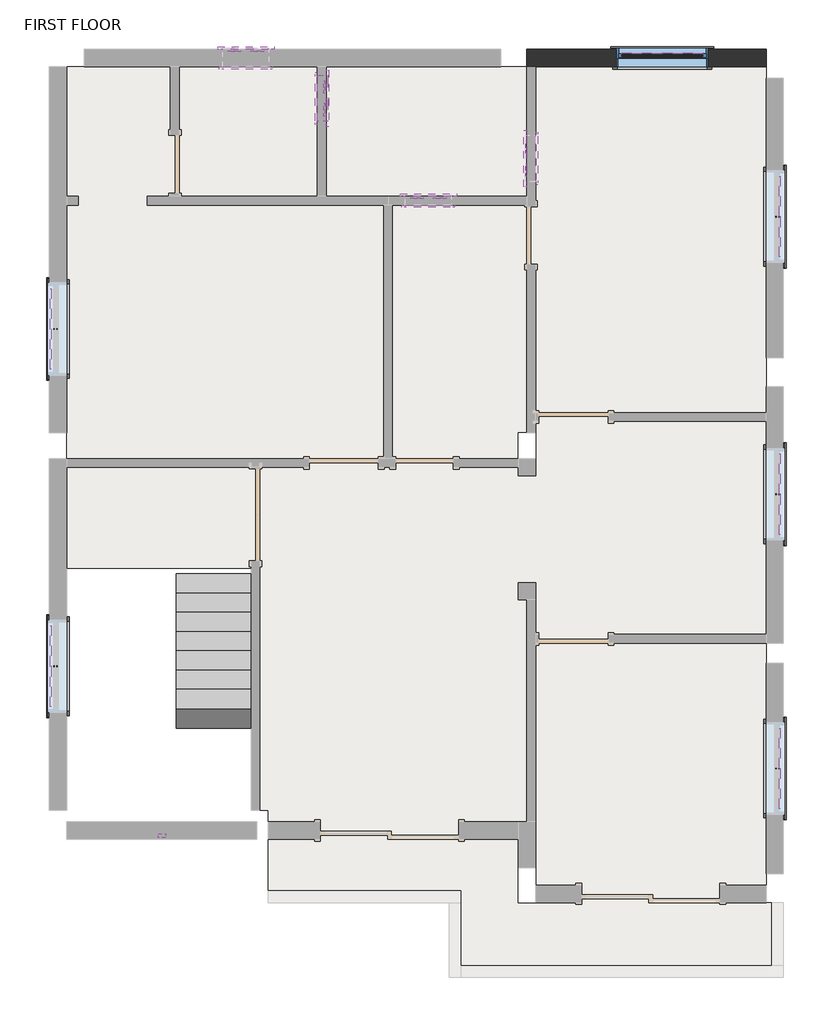
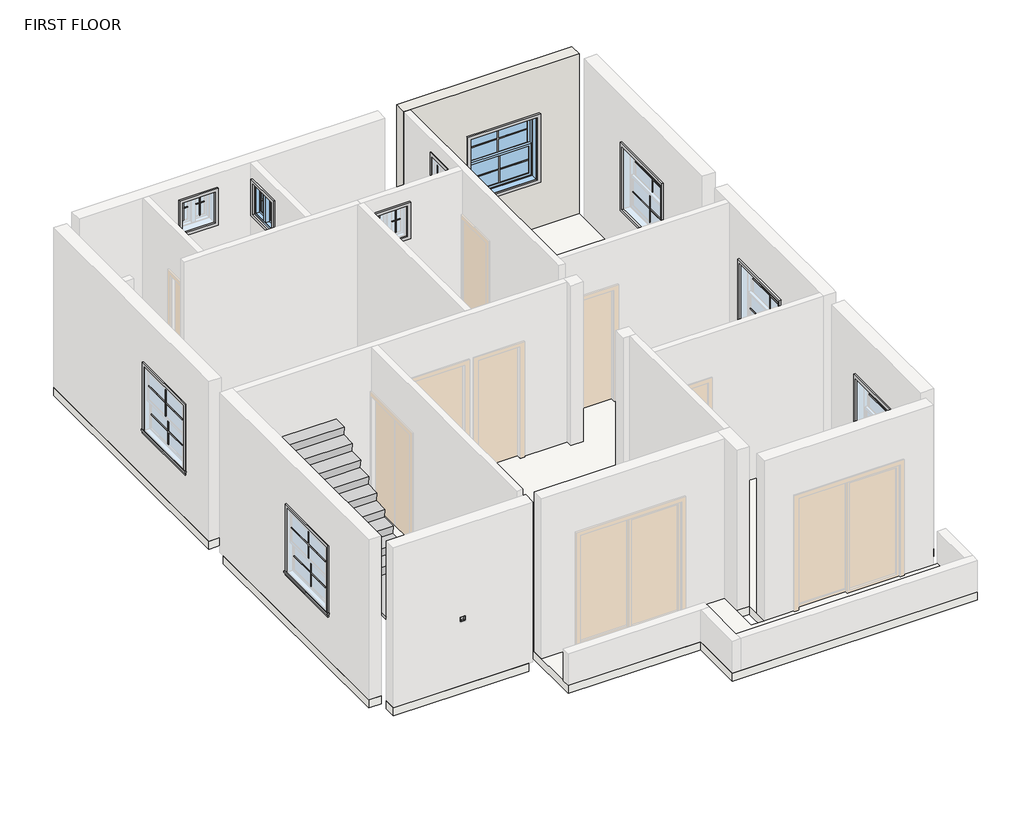
# One storey, part 2 of 2: 40 proxies, 2 windows, 1 light fixture, 1 slab, 1 stair flight, 1 wall.
"""IFC4 building model written with IfcOpenShell, lengths in millimetres."""

from ifc_helpers import new_model, si_unit, frame, origin, place, context, project, spatial, polyline, outline, extrude, faceted_brep, transform, mapped, element, save
from components import muntin_pattern_2x2_muntin_pattern_2x2_1e1a1b39, muntin_pattern_2x2_muntin_pattern_2x2_0961b91c, muntin_pattern_2x2_muntin_pattern_2x2_cae9449b, trim_window_exterior_flat_with_sill_7cfdd449, trim_window_exterior_flat_with_sill_858dc10d, trim_window_interior_flat_picture_frame_f1e0b15b, trim_window_interior_flat_picture_frame_3927330c, light_fixture_da35b629, window_casement_double_2_x2_e4709907, window_double_hung_4_x4_ec8efb0e

model = new_model("IFC4")

# Units and contexts
model_context = context("Model", 3, world=origin())
ifc_project = project(units=[si_unit("LENGTHUNIT", "METRE", prefix="MILLI")], contexts=[model_context])

# Site, building, storey
site = spatial("IfcSite", under=ifc_project)
building = spatial("IfcBuilding", under=site)
storey = spatial("IfcBuildingStorey", under=building, Name="FIRST FLOOR", Elevation=3200.4)

# Proxies
placement = place(None, origin())
muntin_pattern_2x2_muntin_pattern_2x2_shape = muntin_pattern_2x2_muntin_pattern_2x2_1e1a1b39(model_context)
element("IfcBuildingElementProxy", 1, Name="Muntin Pattern_2x2 : Muntin Pattern_2x2", ObjectType="Muntin Pattern_2x2 : Muntin Pattern_2x2", at=placement, inside=storey, context=model_context, shape_type="MappedRepresentation", body=[
    mapped(muntin_pattern_2x2_muntin_pattern_2x2_shape, transform((-12856.4959734, 734.3170657, 4746.625), x_axis=(0.0, 1.0, 0.0), y_axis=(-1.0, 0.0, 0.0), z_axis=(0.0, 0.0, 1.0))),
])
element("IfcBuildingElementProxy", 2, Name="Muntin Pattern_2x2 : Muntin Pattern_2x2", ObjectType="Muntin Pattern_2x2 : Muntin Pattern_2x2", at=placement, inside=storey, context=model_context, shape_type="MappedRepresentation", body=[
    mapped(muntin_pattern_2x2_muntin_pattern_2x2_shape, transform((-12812.0459734, 734.3170657, 4191.0), x_axis=(0.0, 1.0, 0.0), y_axis=(-1.0, 0.0, 0.0), z_axis=(0.0, 0.0, 1.0))),
])
element("IfcBuildingElementProxy", 3, Name="Muntin Pattern_2x2 : Muntin Pattern_2x2", ObjectType="Muntin Pattern_2x2 : Muntin Pattern_2x2", at=placement, inside=storey, context=model_context, shape_type="MappedRepresentation", body=[
    mapped(muntin_pattern_2x2_muntin_pattern_2x2_shape, transform((-12856.4959734, 5192.0170657, 4746.625), x_axis=(0.0, 1.0, 0.0), y_axis=(-1.0, 0.0, 0.0), z_axis=(0.0, 0.0, 1.0))),
])
element("IfcBuildingElementProxy", 4, Name="Muntin Pattern_2x2 : Muntin Pattern_2x2", ObjectType="Muntin Pattern_2x2 : Muntin Pattern_2x2", at=placement, inside=storey, context=model_context, shape_type="MappedRepresentation", body=[
    mapped(muntin_pattern_2x2_muntin_pattern_2x2_shape, transform((-12812.0459734, 5192.0170657, 4191.0), x_axis=(0.0, 1.0, 0.0), y_axis=(-1.0, 0.0, 0.0), z_axis=(0.0, 0.0, 1.0))),
])
element("IfcBuildingElementProxy", 5, Name="Muntin Pattern_2x2 : Muntin Pattern_2x2", ObjectType="Muntin Pattern_2x2 : Muntin Pattern_2x2", at=placement, inside=storey, context=model_context, shape_type="MappedRepresentation", body=[
    mapped(muntin_pattern_2x2_muntin_pattern_2x2_shape, transform((-4788.8209734, 8852.7920657, 4746.625), x_axis=(1.0, 0.0, 0.0), y_axis=(0.0, 1.0, 0.0), z_axis=(0.0, 0.0, 1.0))),
])
element("IfcBuildingElementProxy", 6, Name="Muntin Pattern_2x2 : Muntin Pattern_2x2", ObjectType="Muntin Pattern_2x2 : Muntin Pattern_2x2", at=placement, inside=storey, context=model_context, shape_type="MappedRepresentation", body=[
    mapped(muntin_pattern_2x2_muntin_pattern_2x2_shape, transform((-4788.8209734, 8808.3420657, 4191.0), x_axis=(1.0, 0.0, 0.0), y_axis=(0.0, 1.0, 0.0), z_axis=(0.0, 0.0, 1.0))),
])
element("IfcBuildingElementProxy", 7, Name="Muntin Pattern_2x2 : Muntin Pattern_2x2", ObjectType="Muntin Pattern_2x2 : Muntin Pattern_2x2", at=placement, inside=storey, context=model_context, shape_type="MappedRepresentation", body=[
    mapped(muntin_pattern_2x2_muntin_pattern_2x2_shape, transform((-3223.5459734, 6677.9170657, 4746.625), x_axis=(0.0, -1.0, 0.0), y_axis=(1.0, 0.0, 0.0), z_axis=(0.0, 0.0, 1.0))),
])
element("IfcBuildingElementProxy", 8, Name="Muntin Pattern_2x2 : Muntin Pattern_2x2", ObjectType="Muntin Pattern_2x2 : Muntin Pattern_2x2", at=placement, inside=storey, context=model_context, shape_type="MappedRepresentation", body=[
    mapped(muntin_pattern_2x2_muntin_pattern_2x2_shape, transform((-3267.9959734, 6677.9170657, 4191.0), x_axis=(0.0, -1.0, 0.0), y_axis=(1.0, 0.0, 0.0), z_axis=(0.0, 0.0, 1.0))),
])
element("IfcBuildingElementProxy", 9, Name="Muntin Pattern_2x2 : Muntin Pattern_2x2", ObjectType="Muntin Pattern_2x2 : Muntin Pattern_2x2", at=placement, inside=storey, context=model_context, shape_type="MappedRepresentation", body=[
    mapped(muntin_pattern_2x2_muntin_pattern_2x2_shape, transform((-3223.5459734, 3007.6170657, 4746.625), x_axis=(0.0, -1.0, 0.0), y_axis=(1.0, 0.0, 0.0), z_axis=(0.0, 0.0, 1.0))),
])
element("IfcBuildingElementProxy", 10, Name="Muntin Pattern_2x2 : Muntin Pattern_2x2", ObjectType="Muntin Pattern_2x2 : Muntin Pattern_2x2", at=placement, inside=storey, context=model_context, shape_type="MappedRepresentation", body=[
    mapped(muntin_pattern_2x2_muntin_pattern_2x2_shape, transform((-3267.9959734, 3007.6170657, 4191.0), x_axis=(0.0, -1.0, 0.0), y_axis=(1.0, 0.0, 0.0), z_axis=(0.0, 0.0, 1.0))),
])
element("IfcBuildingElementProxy", 11, Name="Muntin Pattern_2x2 : Muntin Pattern_2x2", ObjectType="Muntin Pattern_2x2 : Muntin Pattern_2x2", at=placement, inside=storey, context=model_context, shape_type="MappedRepresentation", body=[
    mapped(muntin_pattern_2x2_muntin_pattern_2x2_shape, transform((-3223.5459734, -618.2329343, 4746.625), x_axis=(0.0, -1.0, 0.0), y_axis=(1.0, 0.0, 0.0), z_axis=(0.0, 0.0, 1.0))),
])
element("IfcBuildingElementProxy", 12, Name="Muntin Pattern_2x2 : Muntin Pattern_2x2", ObjectType="Muntin Pattern_2x2 : Muntin Pattern_2x2", at=placement, inside=storey, context=model_context, shape_type="MappedRepresentation", body=[
    mapped(muntin_pattern_2x2_muntin_pattern_2x2_shape, transform((-3267.9959734, -618.2329343, 4191.0), x_axis=(0.0, -1.0, 0.0), y_axis=(1.0, 0.0, 0.0), z_axis=(0.0, 0.0, 1.0))),
])
muntin_pattern_2x2_muntin_pattern_2x2_2_shape = muntin_pattern_2x2_muntin_pattern_2x2_0961b91c(model_context)
element("IfcBuildingElementProxy", 13, Name="Muntin Pattern_2x2 : Muntin Pattern_2x2", ObjectType="Muntin Pattern_2x2 : Muntin Pattern_2x2", at=placement, inside=storey, context=model_context, shape_type="MappedRepresentation", body=[
    mapped(muntin_pattern_2x2_muntin_pattern_2x2_2_shape, transform((-8032.0834734, 6935.0920657, 5403.85), x_axis=(1.0, 0.0, 0.0), y_axis=(0.0, 1.0, 0.0), z_axis=(0.0, 0.0, 1.0))),
])
element("IfcBuildingElementProxy", 14, Name="Muntin Pattern_2x2 : Muntin Pattern_2x2", ObjectType="Muntin Pattern_2x2 : Muntin Pattern_2x2", at=placement, inside=storey, context=model_context, shape_type="MappedRepresentation", body=[
    mapped(muntin_pattern_2x2_muntin_pattern_2x2_2_shape, transform((-9243.3459734, 8390.8295657, 5403.85), x_axis=(0.0, -1.0, 0.0), y_axis=(1.0, 0.0, 0.0), z_axis=(0.0, 0.0, 1.0))),
])
element("IfcBuildingElementProxy", 15, Name="Muntin Pattern_2x2 : Muntin Pattern_2x2", ObjectType="Muntin Pattern_2x2 : Muntin Pattern_2x2", at=placement, inside=storey, context=model_context, shape_type="MappedRepresentation", body=[
    mapped(muntin_pattern_2x2_muntin_pattern_2x2_2_shape, transform((-10445.0834734, 8878.1920657, 5403.85), x_axis=(1.0, 0.0, 0.0), y_axis=(0.0, 1.0, 0.0), z_axis=(0.0, 0.0, 1.0))),
])
element("IfcBuildingElementProxy", 16, Name="Muntin Pattern_2x2 : Muntin Pattern_2x2", ObjectType="Muntin Pattern_2x2 : Muntin Pattern_2x2", at=placement, inside=storey, context=model_context, shape_type="MappedRepresentation", body=[
    mapped(muntin_pattern_2x2_muntin_pattern_2x2_2_shape, transform((-6569.9959734, 7295.4545657, 5403.85), x_axis=(0.0, 1.0, 0.0), y_axis=(-1.0, 0.0, 0.0), z_axis=(0.0, 0.0, 1.0))),
])
muntin_pattern_2x2_muntin_pattern_2x2_3_shape = muntin_pattern_2x2_muntin_pattern_2x2_cae9449b(model_context)
element("IfcBuildingElementProxy", 17, Name="Muntin Pattern_2x2 : Muntin Pattern_2x2", ObjectType="Muntin Pattern_2x2 : Muntin Pattern_2x2", at=placement, inside=storey, context=model_context, shape_type="MappedRepresentation", body=[
    mapped(muntin_pattern_2x2_muntin_pattern_2x2_3_shape, transform((-7730.4584734, 6935.0920657, 5403.85), x_axis=(-1.0, 0.0, 0.0), y_axis=(0.0, -1.0, 0.0), z_axis=(0.0, 0.0, 1.0))),
])
element("IfcBuildingElementProxy", 18, Name="Muntin Pattern_2x2 : Muntin Pattern_2x2", ObjectType="Muntin Pattern_2x2 : Muntin Pattern_2x2", at=placement, inside=storey, context=model_context, shape_type="MappedRepresentation", body=[
    mapped(muntin_pattern_2x2_muntin_pattern_2x2_3_shape, transform((-9243.3459734, 8089.2045657, 5403.85), x_axis=(0.0, 1.0, 0.0), y_axis=(-1.0, 0.0, 0.0), z_axis=(0.0, 0.0, 1.0))),
])
element("IfcBuildingElementProxy", 19, Name="Muntin Pattern_2x2 : Muntin Pattern_2x2", ObjectType="Muntin Pattern_2x2 : Muntin Pattern_2x2", at=placement, inside=storey, context=model_context, shape_type="MappedRepresentation", body=[
    mapped(muntin_pattern_2x2_muntin_pattern_2x2_3_shape, transform((-10143.4584734, 8878.1920657, 5403.85), x_axis=(-1.0, 0.0, 0.0), y_axis=(0.0, -1.0, 0.0), z_axis=(0.0, 0.0, 1.0))),
])
element("IfcBuildingElementProxy", 20, Name="Muntin Pattern_2x2 : Muntin Pattern_2x2", ObjectType="Muntin Pattern_2x2 : Muntin Pattern_2x2", at=placement, inside=storey, context=model_context, shape_type="MappedRepresentation", body=[
    mapped(muntin_pattern_2x2_muntin_pattern_2x2_3_shape, transform((-6569.9959734, 7597.0795657, 5403.85), x_axis=(0.0, -1.0, 0.0), y_axis=(1.0, 0.0, 0.0), z_axis=(0.0, 0.0, 1.0))),
])
trim_window_exterior_flat_with_sill_shape = trim_window_exterior_flat_with_sill_7cfdd449(model_context)
element("IfcBuildingElementProxy", 21, Name="Trim-Window-Exterior-Flat : with Sill", ObjectType="Trim-Window-Exterior-Flat : with Sill", at=placement, inside=storey, context=model_context, shape_type="MappedRepresentation", body=[
    mapped(trim_window_exterior_flat_with_sill_shape, transform((-12891.4209734, 734.3170657, 5334.0), x_axis=(0.0, -1.0, 0.0), y_axis=(0.0, 0.0, 1.0), z_axis=(-1.0, 0.0, 0.0))),
])
element("IfcBuildingElementProxy", 22, Name="Trim-Window-Exterior-Flat : with Sill", ObjectType="Trim-Window-Exterior-Flat : with Sill", at=placement, inside=storey, context=model_context, shape_type="MappedRepresentation", body=[
    mapped(trim_window_exterior_flat_with_sill_shape, transform((-12891.4209734, 5192.0170657, 5334.0), x_axis=(0.0, -1.0, 0.0), y_axis=(0.0, 0.0, 1.0), z_axis=(-1.0, 0.0, 0.0))),
])
element("IfcBuildingElementProxy", 23, Name="Trim-Window-Exterior-Flat : with Sill", ObjectType="Trim-Window-Exterior-Flat : with Sill", at=placement, inside=storey, context=model_context, shape_type="MappedRepresentation", body=[
    mapped(trim_window_exterior_flat_with_sill_shape, transform((-4788.8209734, 8887.7170657, 5334.0), x_axis=(-1.0, 0.0, 0.0), y_axis=(0.0, 0.0, 1.0), z_axis=(0.0, 1.0, 0.0))),
])
element("IfcBuildingElementProxy", 24, Name="Trim-Window-Exterior-Flat : with Sill", ObjectType="Trim-Window-Exterior-Flat : with Sill", at=placement, inside=storey, context=model_context, shape_type="MappedRepresentation", body=[
    mapped(trim_window_exterior_flat_with_sill_shape, transform((-3188.6209734, 6677.9170657, 5334.0), x_axis=(0.0, 1.0, 0.0), y_axis=(0.0, 0.0, 1.0), z_axis=(1.0, 0.0, 0.0))),
])
element("IfcBuildingElementProxy", 25, Name="Trim-Window-Exterior-Flat : with Sill", ObjectType="Trim-Window-Exterior-Flat : with Sill", at=placement, inside=storey, context=model_context, shape_type="MappedRepresentation", body=[
    mapped(trim_window_exterior_flat_with_sill_shape, transform((-3188.6209734, 3007.6170657, 5334.0), x_axis=(0.0, 1.0, 0.0), y_axis=(0.0, 0.0, 1.0), z_axis=(1.0, 0.0, 0.0))),
])
element("IfcBuildingElementProxy", 26, Name="Trim-Window-Exterior-Flat : with Sill", ObjectType="Trim-Window-Exterior-Flat : with Sill", at=placement, inside=storey, context=model_context, shape_type="MappedRepresentation", body=[
    mapped(trim_window_exterior_flat_with_sill_shape, transform((-3188.6209734, -618.2329343, 5334.0), x_axis=(0.0, 1.0, 0.0), y_axis=(0.0, 0.0, 1.0), z_axis=(1.0, 0.0, 0.0))),
])
trim_window_exterior_flat_with_sill_2_shape = trim_window_exterior_flat_with_sill_858dc10d(model_context)
element("IfcBuildingElementProxy", 27, Name="Trim-Window-Exterior-Flat : with Sill", ObjectType="Trim-Window-Exterior-Flat : with Sill", at=placement, inside=storey, context=model_context, shape_type="MappedRepresentation", body=[
    mapped(trim_window_exterior_flat_with_sill_2_shape, transform((-7881.2709734, 6944.6170657, 5943.6), x_axis=(-1.0, 0.0, 0.0), y_axis=(0.0, 0.0, 1.0), z_axis=(0.0, 1.0, 0.0))),
])
element("IfcBuildingElementProxy", 28, Name="Trim-Window-Exterior-Flat : with Sill", ObjectType="Trim-Window-Exterior-Flat : with Sill", at=placement, inside=storey, context=model_context, shape_type="MappedRepresentation", body=[
    mapped(trim_window_exterior_flat_with_sill_2_shape, transform((-9233.8209734, 8240.0170657, 5943.6), x_axis=(0.0, 1.0, 0.0), y_axis=(0.0, 0.0, 1.0), z_axis=(1.0, 0.0, 0.0))),
])
element("IfcBuildingElementProxy", 29, Name="Trim-Window-Exterior-Flat : with Sill", ObjectType="Trim-Window-Exterior-Flat : with Sill", at=placement, inside=storey, context=model_context, shape_type="MappedRepresentation", body=[
    mapped(trim_window_exterior_flat_with_sill_2_shape, transform((-10294.2709734, 8887.7170657, 5943.6), x_axis=(-1.0, 0.0, 0.0), y_axis=(0.0, 0.0, 1.0), z_axis=(0.0, 1.0, 0.0))),
])
element("IfcBuildingElementProxy", 30, Name="Trim-Window-Exterior-Flat : with Sill", ObjectType="Trim-Window-Exterior-Flat : with Sill", at=placement, inside=storey, context=model_context, shape_type="MappedRepresentation", body=[
    mapped(trim_window_exterior_flat_with_sill_2_shape, transform((-6579.5209734, 7446.2670657, 5943.6), x_axis=(0.0, -1.0, 0.0), y_axis=(0.0, 0.0, 1.0), z_axis=(-1.0, 0.0, 0.0))),
])
trim_window_interior_flat_picture_frame_shape = trim_window_interior_flat_picture_frame_f1e0b15b(model_context)
element("IfcBuildingElementProxy", 31, Name="Trim-Window-Interior-Flat : Picture Frame", ObjectType="Trim-Window-Interior-Flat : Picture Frame", at=placement, inside=storey, context=model_context, shape_type="MappedRepresentation", body=[
    mapped(trim_window_interior_flat_picture_frame_shape, transform((-12662.8209734, 734.3170657, 5334.0), x_axis=(0.0, 1.0, 0.0), y_axis=(0.0, 0.0, 1.0), z_axis=(1.0, 0.0, 0.0))),
])
element("IfcBuildingElementProxy", 32, Name="Trim-Window-Interior-Flat : Picture Frame", ObjectType="Trim-Window-Interior-Flat : Picture Frame", at=placement, inside=storey, context=model_context, shape_type="MappedRepresentation", body=[
    mapped(trim_window_interior_flat_picture_frame_shape, transform((-12662.8209734, 5192.0170657, 5334.0), x_axis=(0.0, 1.0, 0.0), y_axis=(0.0, 0.0, 1.0), z_axis=(1.0, 0.0, 0.0))),
])
element("IfcBuildingElementProxy", 33, Name="Trim-Window-Interior-Flat : Picture Frame", ObjectType="Trim-Window-Interior-Flat : Picture Frame", at=placement, inside=storey, context=model_context, shape_type="MappedRepresentation", body=[
    mapped(trim_window_interior_flat_picture_frame_shape, transform((-4788.8209734, 8659.1170657, 5334.0), x_axis=(1.0, 0.0, 0.0), y_axis=(0.0, 0.0, 1.0), z_axis=(0.0, -1.0, 0.0))),
])
element("IfcBuildingElementProxy", 34, Name="Trim-Window-Interior-Flat : Picture Frame", ObjectType="Trim-Window-Interior-Flat : Picture Frame", at=placement, inside=storey, context=model_context, shape_type="MappedRepresentation", body=[
    mapped(trim_window_interior_flat_picture_frame_shape, transform((-3417.2209734, 6677.9170657, 5334.0), x_axis=(0.0, -1.0, 0.0), y_axis=(0.0, 0.0, 1.0), z_axis=(-1.0, 0.0, 0.0))),
])
element("IfcBuildingElementProxy", 35, Name="Trim-Window-Interior-Flat : Picture Frame", ObjectType="Trim-Window-Interior-Flat : Picture Frame", at=placement, inside=storey, context=model_context, shape_type="MappedRepresentation", body=[
    mapped(trim_window_interior_flat_picture_frame_shape, transform((-3417.2209734, 3007.6170657, 5334.0), x_axis=(0.0, -1.0, 0.0), y_axis=(0.0, 0.0, 1.0), z_axis=(-1.0, 0.0, 0.0))),
])
element("IfcBuildingElementProxy", 36, Name="Trim-Window-Interior-Flat : Picture Frame", ObjectType="Trim-Window-Interior-Flat : Picture Frame", at=placement, inside=storey, context=model_context, shape_type="MappedRepresentation", body=[
    mapped(trim_window_interior_flat_picture_frame_shape, transform((-3417.2209734, -618.2329343, 5334.0), x_axis=(0.0, -1.0, 0.0), y_axis=(0.0, 0.0, 1.0), z_axis=(-1.0, 0.0, 0.0))),
])
trim_window_interior_flat_picture_frame_2_shape = trim_window_interior_flat_picture_frame_3927330c(model_context)
element("IfcBuildingElementProxy", 37, Name="Trim-Window-Interior-Flat : Picture Frame", ObjectType="Trim-Window-Interior-Flat : Picture Frame", at=placement, inside=storey, context=model_context, shape_type="MappedRepresentation", body=[
    mapped(trim_window_interior_flat_picture_frame_2_shape, transform((-7881.2709734, 6830.3170657, 5943.6), x_axis=(1.0, 0.0, 0.0), y_axis=(0.0, 0.0, 1.0), z_axis=(0.0, -1.0, 0.0))),
])
element("IfcBuildingElementProxy", 38, Name="Trim-Window-Interior-Flat : Picture Frame", ObjectType="Trim-Window-Interior-Flat : Picture Frame", at=placement, inside=storey, context=model_context, shape_type="MappedRepresentation", body=[
    mapped(trim_window_interior_flat_picture_frame_2_shape, transform((-9348.1209734, 8240.0170657, 5943.6), x_axis=(0.0, -1.0, 0.0), y_axis=(0.0, 0.0, 1.0), z_axis=(-1.0, 0.0, 0.0))),
])
element("IfcBuildingElementProxy", 39, Name="Trim-Window-Interior-Flat : Picture Frame", ObjectType="Trim-Window-Interior-Flat : Picture Frame", at=placement, inside=storey, context=model_context, shape_type="MappedRepresentation", body=[
    mapped(trim_window_interior_flat_picture_frame_2_shape, transform((-10294.2709734, 8659.1170657, 5943.6), x_axis=(1.0, 0.0, 0.0), y_axis=(0.0, 0.0, 1.0), z_axis=(0.0, -1.0, 0.0))),
])
element("IfcBuildingElementProxy", 40, Name="Trim-Window-Interior-Flat : Picture Frame", ObjectType="Trim-Window-Interior-Flat : Picture Frame", at=placement, inside=storey, context=model_context, shape_type="MappedRepresentation", body=[
    mapped(trim_window_interior_flat_picture_frame_2_shape, transform((-6465.2209734, 7446.2670657, 5943.6), x_axis=(0.0, 1.0, 0.0), y_axis=(0.0, 0.0, 1.0), z_axis=(1.0, 0.0, 0.0))),
])

# Light fixture
light_fixture_shape = light_fixture_da35b629(model_context)
element("IfcLightFixture", 41, at=placement, inside=storey, context=model_context, shape_type="MappedRepresentation", body=[
    mapped(light_fixture_shape, transform((-11441.8766361, -1437.3829343, 2452.7878889), x_axis=(-1.0, 0.0, 0.0), y_axis=(0.0, -1.0, 0.0), z_axis=(0.0, 0.0, 1.0))),
])

# Slab
element("IfcSlab", 42, ObjectType="6\"", at=placement, inside=storey, context=model_context, shape_type="SweptSolid", body=[
    extrude(outline(polyline([(-3188.6209734, -3380.4829343), (-7608.2209734, -3380.4829343), (-7608.2209734, -2389.8829343), (-9995.8209734, -2389.8829343), (-9995.8209734, -1170.6829343), (-10224.4209734, -1170.6829343), (-10224.4209734, 2029.7170657), (-12662.8209734, 2029.7170657), (-12662.8209734, -1170.6829343), (-12891.4209734, -1170.6829343), (-12891.4209734, 3363.2170657), (-12662.8209734, 3363.2170657), (-12662.8209734, 3820.4170657), (-12891.4209734, 3820.4170657), (-12891.4209734, 8659.1170657), (-12434.2209734, 8659.1170657), (-12434.2209734, 8887.7170657), (-6922.4209734, 8887.7170657), (-6922.4209734, 8659.1170657), (-6465.2209734, 8659.1170657), (-6465.2209734, 8887.7170657), (-3417.2209734, 8887.7170657), (-3417.2209734, 8506.7170657), (-3188.6209734, 8506.7170657), (-3188.6209734, 4811.0170657), (-3417.2209734, 4811.0170657), (-3417.2209734, 4430.0170657), (-3188.6209734, 4430.0170657), (-3188.6209734, 1153.4170657), (-3417.2209734, 1153.4170657), (-3417.2209734, 772.4170657), (-3188.6209734, 772.4170657), (-3188.6209734, -1746.9354412), (-3188.6209734, -2008.8829343), (-3417.2209734, -2008.8829343), (-3417.2209734, -2389.8829343), (-3188.6209734, -2389.8829343), (-3188.6209734, -3380.4829343)]), holes=[polyline([(-6693.8209734, -1932.6829343), (-6693.8209734, -2389.8829343), (-6465.2209734, -2389.8829343), (-6465.2209734, -1932.6829343), (-6693.8209734, -1932.6829343)]), polyline([(-6693.8209734, 3820.4170657), (-6693.8209734, 3363.2170657), (-6465.2209734, 3363.2170657), (-6465.2209734, 3820.4170657), (-6693.8209734, 3820.4170657)])]), frame((0.0, 0.0, 3048.0), z_axis=(0.0, 0.0, 1.0), x_axis=(1.0, 0.0, 0.0)), (0.0, 0.0, 1.0), 152.4),
    extrude(outline(polyline([(-12662.8209734, -1323.0829343), (-10224.4209734, -1323.0829343), (-10224.4209734, -1551.6829343), (-12662.8209734, -1551.6829343), (-12662.8209734, -1323.0829343)])), frame((0.0, 0.0, 3048.0), z_axis=(0.0, 0.0, 1.0), x_axis=(1.0, 0.0, 0.0)), (0.0, 0.0, 1.0), 152.4),
])

# Stair flight
element("IfcStairFlight", 43, ObjectType="3/4\" Nosing", at=placement, inside=storey, context=model_context, shape_type="Brep", body=[
    faceted_brep([(-10224.4209734, 1953.5170657, 3360.42), (-11215.0209734, 1953.5170657, 3360.42), (-11215.0209734, 1680.4670657, 3360.42), (-10224.4209734, 1680.4670657, 3360.42), (-10224.4209734, 1680.4670657, 3285.3690172), (-10224.4209734, 1815.3385215, 3200.4), (-10224.4209734, 1934.4670657, 3200.4), (-11215.0209734, 1934.4670657, 3200.4), (-11215.0209734, 1815.3385215, 3200.4), (-11215.0209734, 1680.4670657, 3285.3690172), (-10224.4209734, 1699.5170657, 3520.44), (-11215.0209734, 1699.5170657, 3520.44), (-11215.0209734, 1426.4670657, 3520.44), (-10224.4209734, 1426.4670657, 3520.44), (-10224.4209734, 1426.4670657, 3445.3890172), (-11215.0209734, 1426.4670657, 3445.3890172), (-10224.4209734, 1445.5170657, 3680.46), (-11215.0209734, 1445.5170657, 3680.46), (-11215.0209734, 1172.4670657, 3680.46), (-10224.4209734, 1172.4670657, 3680.46), (-10224.4209734, 1172.4670657, 3605.4090172), (-11215.0209734, 1172.4670657, 3605.4090172), (-10224.4209734, 1191.5170657, 3840.48), (-11215.0209734, 1191.5170657, 3840.48), (-11215.0209734, 918.4670657, 3840.48), (-10224.4209734, 918.4670657, 3840.48), (-10224.4209734, 918.4670657, 3765.4290172), (-11215.0209734, 918.4670657, 3765.4290172), (-10224.4209734, 937.5170657, 4000.5), (-11215.0209734, 937.5170657, 4000.5), (-11215.0209734, 664.4670657, 4000.5), (-10224.4209734, 664.4670657, 4000.5), (-10224.4209734, 664.4670657, 3925.4490172), (-11215.0209734, 664.4670657, 3925.4490172), (-10224.4209734, 683.5170657, 4160.52), (-11215.0209734, 683.5170657, 4160.52), (-11215.0209734, 410.4670657, 4160.52), (-10224.4209734, 410.4670657, 4160.52), (-10224.4209734, 410.4670657, 4085.4690172), (-11215.0209734, 410.4670657, 4085.4690172), (-10224.4209734, 429.5170657, 4320.54), (-11215.0209734, 429.5170657, 4320.54), (-11215.0209734, 156.4670657, 4320.54), (-10224.4209734, 156.4670657, 4320.54), (-10224.4209734, 156.4670657, 4245.4890172), (-11215.0209734, 156.4670657, 4245.4890172), (-10224.4209734, 175.5170657, 4480.56), (-11215.0209734, 175.5170657, 4480.56), (-11215.0209734, -97.5329343, 4480.56), (-10224.4209734, -97.5329343, 4480.56), (-10224.4209734, -97.5329343, 4405.5090172), (-11215.0209734, -97.5329343, 4405.5090172), (-10224.4209734, -78.4829343, 4640.58), (-11215.0209734, -78.4829343, 4640.58), (-11215.0209734, -351.5329343, 4640.58), (-10224.4209734, -351.5329343, 4640.58), (-10224.4209734, -351.5329343, 4565.5290172), (-11215.0209734, -623.8678277, 4737.1), (-11215.0209734, -340.0424581, 4737.1), (-12662.8209734, -313.4329343, 4800.6), (-12662.8209734, -1323.0829343, 4800.6), (-10224.4209734, -1323.0829343, 4800.6), (-10224.4209734, -623.8678277, 4800.6), (-10224.4209734, -332.4829343, 4800.6), (-11215.0209734, -332.4829343, 4800.6), (-11672.2209734, -332.4829343, 4800.6), (-11672.2209734, -313.4329343, 4800.6), (-12662.8209734, -313.4329343, 4737.1), (-12662.8209734, -1323.0829343, 4737.1), (-10224.4209734, -1323.0829343, 4737.1), (-10224.4209734, -623.8678277, 4737.1), (-11215.0209734, -332.4829343, 4737.1), (-11672.2209734, -332.4829343, 4737.1), (-11672.2209734, -313.4329343, 4737.1), (-12662.8209734, -332.4829343, 4960.62), (-11672.2209734, -332.4829343, 4960.62), (-11672.2209734, -295.0980409, 4960.62), (-11672.2209734, -59.4329343, 4960.62), (-12662.8209734, -59.4329343, 4960.62), (-12662.8209734, -295.0980409, 4960.62), (-12662.8209734, -59.4329343, 4885.5690172), (-12662.8209734, -295.0980409, 4737.1), (-11672.2209734, -295.0980409, 4737.1), (-11672.2209734, -59.4329343, 4885.5690172), (-12662.8209734, -78.4829343, 5120.64), (-11672.2209734, -78.4829343, 5120.64), (-11672.2209734, 194.5670657, 5120.64), (-12662.8209734, 194.5670657, 5120.64), (-12662.8209734, 194.5670657, 5045.5890172), (-11672.2209734, 194.5670657, 5045.5890172), (-12662.8209734, 175.5170657, 5280.66), (-11672.2209734, 175.5170657, 5280.66), (-11672.2209734, 448.5670657, 5280.66), (-12662.8209734, 448.5670657, 5280.66), (-12662.8209734, 448.5670657, 5205.6090172), (-11672.2209734, 448.5670657, 5205.6090172), (-12662.8209734, 429.5170657, 5440.68), (-11672.2209734, 429.5170657, 5440.68), (-11672.2209734, 702.5670657, 5440.68), (-12662.8209734, 702.5670657, 5440.68), (-12662.8209734, 702.5670657, 5365.6290172), (-11672.2209734, 702.5670657, 5365.6290172), (-12662.8209734, 683.5170657, 5600.7), (-11672.2209734, 683.5170657, 5600.7), (-11672.2209734, 956.5670657, 5600.7), (-12662.8209734, 956.5670657, 5600.7), (-12662.8209734, 956.5670657, 5525.6490172), (-11672.2209734, 956.5670657, 5525.6490172), (-12662.8209734, 937.5170657, 5760.72), (-11672.2209734, 937.5170657, 5760.72), (-11672.2209734, 1210.5670657, 5760.72), (-12662.8209734, 1210.5670657, 5760.72), (-12662.8209734, 1210.5670657, 5685.6690172), (-11672.2209734, 1210.5670657, 5685.6690172), (-12662.8209734, 1191.5170657, 5920.74), (-11672.2209734, 1191.5170657, 5920.74), (-11672.2209734, 1464.5670657, 5920.74), (-12662.8209734, 1464.5670657, 5920.74), (-12662.8209734, 1464.5670657, 5845.6890172), (-11672.2209734, 1464.5670657, 5845.6890172), (-12662.8209734, 1445.5170657, 6080.76), (-11672.2209734, 1445.5170657, 6080.76), (-11672.2209734, 1718.5670657, 6080.76), (-12662.8209734, 1718.5670657, 6080.76), (-12662.8209734, 1718.5670657, 6005.7090172), (-11672.2209734, 1718.5670657, 6005.7090172), (-12662.8209734, 1699.5170657, 6240.78), (-11672.2209734, 1699.5170657, 6240.78), (-11672.2209734, 1953.5170657, 6240.78), (-12662.8209734, 1953.5170657, 6240.78), (-12662.8209734, 1953.5170657, 6153.7275172), (-11672.2209734, 1953.5170657, 6153.7275172)], [[[0, 1, 2, 3]], [[0, 3, 4, 5, 6]], [[2, 1, 7, 8, 9]], [[10, 11, 12, 13]], [[10, 13, 14, 4, 3]], [[12, 11, 2, 9, 15]], [[16, 17, 18, 19]], [[16, 19, 20, 14, 13]], [[18, 17, 12, 15, 21]], [[22, 23, 24, 25]], [[22, 25, 26, 20, 19]], [[24, 23, 18, 21, 27]], [[28, 29, 30, 31]], [[28, 31, 32, 26, 25]], [[30, 29, 24, 27, 33]], [[34, 35, 36, 37]], [[34, 37, 38, 32, 31]], [[36, 35, 30, 33, 39]], [[40, 41, 42, 43]], [[40, 43, 44, 38, 37]], [[42, 41, 36, 39, 45]], [[46, 47, 48, 49]], [[46, 49, 50, 44, 43]], [[48, 47, 42, 45, 51]], [[52, 53, 54, 55]], [[52, 55, 56, 50, 49]], [[53, 48, 51, 57, 58, 54]], [[59, 60, 61, 62, 63, 64, 65, 66]], [[60, 59, 67, 68]], [[61, 60, 68, 69]], [[55, 63, 62, 61, 69, 70, 56]], [[64, 58, 71]], [[65, 64, 71, 72]], [[66, 65, 72, 73]], [[74, 75, 76, 77, 78, 79]], [[59, 74, 79, 78, 80, 81, 67]], [[75, 66, 73, 82, 83, 77, 76]], [[84, 85, 86, 87]], [[84, 87, 88, 80, 78]], [[86, 85, 77, 83, 89]], [[90, 91, 92, 93]], [[90, 93, 94, 88, 87]], [[92, 91, 86, 89, 95]], [[96, 97, 98, 99]], [[96, 99, 100, 94, 93]], [[98, 97, 92, 95, 101]], [[102, 103, 104, 105]], [[102, 105, 106, 100, 99]], [[104, 103, 98, 101, 107]], [[108, 109, 110, 111]], [[108, 111, 112, 106, 105]], [[110, 109, 104, 107, 113]], [[114, 115, 116, 117]], [[114, 117, 118, 112, 111]], [[116, 115, 110, 113, 119]], [[120, 121, 122, 123]], [[120, 123, 124, 118, 117]], [[122, 121, 116, 119, 125]], [[1, 0, 6, 7]], [[3, 2, 11, 10]], [[13, 12, 17, 16]], [[19, 18, 23, 22]], [[25, 24, 29, 28]], [[31, 30, 35, 34]], [[37, 36, 41, 40]], [[43, 42, 47, 46]], [[49, 48, 53, 52]], [[55, 54, 58, 64, 63]], [[59, 66, 75, 74]], [[78, 77, 85, 84]], [[87, 86, 91, 90]], [[93, 92, 97, 96]], [[99, 98, 103, 102]], [[105, 104, 109, 108]], [[111, 110, 115, 114]], [[117, 116, 121, 120]], [[126, 127, 128, 129]], [[126, 129, 130, 124, 123]], [[128, 127, 122, 125, 131]], [[129, 128, 131, 130]], [[123, 122, 127, 126]], [[7, 6, 5, 8]], [[70, 57, 51, 45, 39, 33, 27, 21, 15, 9, 8, 5, 4, 14, 20, 26, 32, 38, 44, 50, 56]], [[57, 70, 69, 68, 67, 81, 82, 73, 72, 71, 58]], [[82, 81, 80, 88, 94, 100, 106, 112, 118, 124, 130, 131, 125, 119, 113, 107, 101, 95, 89, 83]]]),
])

# Wall
element("IfcWall", 44, ObjectType="9\"", at=placement, inside=storey, context=model_context, shape_type="Brep", body=[
    faceted_brep([(-6579.5209734, 8659.1170657, 3200.4), (-6465.2209734, 8659.1170657, 3200.4), (-3417.2209734, 8659.1170657, 3200.4), (-3417.2209734, 8659.1170657, 6248.4), (-6465.2209734, 8659.1170657, 6248.4), (-6579.5209734, 8659.1170657, 6248.4), (-5398.4209734, 8659.1170657, 5334.0), (-4179.2209734, 8659.1170657, 5334.0), (-4179.2209734, 8659.1170657, 4114.8), (-5398.4209734, 8659.1170657, 4114.8), (-6579.5209734, 8887.7170657, 3200.4), (-6579.5209734, 8887.7170657, 6248.4), (-6465.2209734, 8887.7170657, 6248.4), (-3417.2209734, 8887.7170657, 6248.4), (-3417.2209734, 8887.7170657, 3200.4), (-6465.2209734, 8887.7170657, 3200.4), (-5398.4209734, 8887.7170657, 5334.0), (-5398.4209734, 8887.7170657, 4114.8), (-4179.2209734, 8887.7170657, 4114.8), (-4179.2209734, 8887.7170657, 5334.0)], [[[0, 1, 2, 3, 4, 5], [6, 7, 8, 9]], [[10, 11, 12, 13, 14, 15], [16, 17, 18, 19]], [[2, 1, 0, 10, 15, 14]], [[3, 2, 14, 13]], [[5, 4, 3, 13, 12, 11]], [[0, 5, 11, 10]], [[17, 16, 6, 9]], [[18, 17, 9, 8]], [[19, 18, 8, 7]], [[16, 19, 7, 6]]]),
])

# Windows
window_casement_double_2_x2_shape = window_casement_double_2_x2_e4709907(model_context)
element("IfcWindow", 45, ObjectType="Window-Casement-Double : 2'X2'", at=placement, inside=storey, context=model_context, shape_type="MappedRepresentation", body=[
    mapped(window_casement_double_2_x2_shape, transform((-9290.9709734, 8240.0170657, 4419.6), x_axis=(0.0, -1.0, 0.0), y_axis=(1.0, 0.0, 0.0), z_axis=(0.0, 0.0, 1.0))),
])
window_double_hung_4_x4_shape = window_double_hung_4_x4_ec8efb0e(model_context)
element("IfcWindow", 46, ObjectType="Window-Double-Hung : 4'X4'", at=placement, inside=storey, context=model_context, shape_type="MappedRepresentation", body=[
    mapped(window_double_hung_4_x4_shape, transform((-4788.8209734, 8773.4170657, 3200.4), x_axis=(1.0, 0.0, 0.0), y_axis=(0.0, 1.0, 0.0), z_axis=(0.0, 0.0, 1.0))),
])

save(model, "model.ifc")

# Revit data of these elements
# Type "Muntin Pattern_2x2 : Muntin Pattern_2x2"
#   Width [instance default] = 4' - 0"
#   Thickness = 0' - 0 1/2"
#   Height [instance default] = 4' - 0"
#   Distance = 0' - 0 3/4"
#   Interior Material [instance default] = none
#   Exterior Material [instance default] = none
#   Default Elevation = 0
# Type "Trim-Window-Exterior-Flat : with Sill"
#   Trim Width = 0' - 2 1/4"
#   Trim Thickness_Picture Frame = 0' - 1 1/4"
#   Trim Thickness_with Sill = 0' - 0 3/4"
#   Sill Thickness = 0' - 1 1/4"
#   Opening Width [instance default] = 2' - 0"
#   Opening Height [instance default] = 3' - 0"
#   Default Elevation = 4' - 0"
#   Sill = yes
#   Picture Frame = no
#   Trim Material [instance default] = none
# Type "Trim-Window-Interior-Flat : Picture Frame"
#   Trim Thickness_Picture Frame = 0' - 1 1/4"
#   Trim Width = 0' - 2 1/4"
#   Trim Thickness_with Sill = 0' - 0 3/4"
#   Sill Thickness = 0' - 1 1/4"
#   Opening Width [instance default] = 2' - 0"
#   Opening Height [instance default] = 3' - 0"
#   Default Elevation = 4' - 0"
#   Sill = no
#   Picture Frame = yes
#   Trim Material [instance default] = none
# Type
#   rahmen dicke = 0' - 0.98819"
#   rahmen breite(okvir) = 0' - 0.55118"
#   rahmen breite = 0' - 1.9685"
#   glas dicke = 0' - 0.82349"
#   abstand von wand (lichtquelle) = 0' - 2.76378"
#   Wattage = 20.16 W
#   Emit from Circle Diameter = 0' - 4.31496"
#   built-in parameter 1150110 = 1 (stored number, unit not read)
#   built-in parameter 1114217 = 1 (stored number, unit not read)
#   built-in parameter 1150109 = 1 (stored number, unit not read)
#   built-in parameter 1150113 = 1 (stored number, unit not read)
#   Lumens = 2994.61 lm
#   built-in parameter 1150115 = 1 (stored number, unit not read)
#   built-in parameter 1150105 = 953.213 (stored number, unit not read)
#   Light Source Symbol Size = 2' - 0"
#   built-in parameter 1150112 = 1 (stored number, unit not read)
#   built-in parameter 1150114 = 1 (stored number, unit not read)
#   built-in parameter 1150107 = 3000 (stored number, unit not read)
#   built-in parameter 1150106 = 9.53213 (stored number, unit not read)
#   built-in parameter 1150104 = 13.8 (stored number, unit not read)
#   built-in parameter 1114218 = 1 (stored number, unit not read)
#   built-in parameter 1150133 = 10 (stored number, unit not read)
#   Emit Shape Visible in Rendering = yes
#   Color Filter = 16744448
#   rahmen material = rahmen material
#   glass material = glas material
#   Dimming Lamp Color Temperature Shift = (empty or 0)
#   Default Elevation = 0
# Type "6\""
#   Assembly Code = "B1010"
#   Function = 0
#   Layers, outside or top first: 0' - 6" no material (function 1)
# Type "9\""
#   Assembly Code = "B2010"
#   Layers, outside or top first: 0' - 9" no material (function 1)
# Type "Window-Casement-Double : 2'X2'"
#   Type Mark = "20"
#   Fire Rating = "0.5h"
#   Assembly Code = "B2020100"
#   Analytic Construction = "Double glazing - domestic"
#   Frame Extension [instance default] = 0' - 0 1/4"
#   Window Inset [instance default] = 0' - 0"
#   Wall Thickness [instance default] = 0' - 6"
#   Interior Wall Closure [instance default] = 0' - 2 1/4"
#   Half Width = 1' - 0"
#   Visual Light Transmittance = 0.81
#   Thermal Resistance (R) = 1.8146 (h·ft²·°F)/BTU
#   Solar Heat Gain Coefficient = 0.76
#   Rough Width = 2' - 0 1/2"
#   Rough Height = 2' - 0 1/2"
#   Height = 2' - 0"
#   Heat Transfer Coefficient (U) = 0.5511 BTU/(h·ft²·°F)
#   Exterior Wall Closure [instance default] = 0' - 1 1/4"
#   Extension Jamb [instance default] = 0' - 2 1/4"
#   Default Sill Height = 3' - 0"
#   Width = 2' - 0"
#   Muntin Visibility = yes
#   Interior Trim Visibility [instance default] = yes
#   Exterior Trim Visibility [instance default] = yes
#   Extension Jamb Visibility [instance default] = yes
#   Interior Trim Material = Wood - Stained
#   Muntin Pattern = Muntin Pattern_2x2 : Muntin Pattern_2x2
#   Interior Trim = Trim-Window-Interior-Flat : Picture Frame
#   Interior Frame Material = Wood - Stained
#   Glass Panel Material = Glass
#   Exterior Trim Material = Clad - White
#   Exterior Trim = Trim-Window-Exterior-Flat : with Sill
#   Exterior Frame Material = Clad - White
#   Wall Closure = (empty or 0)
# Type "Window-Double-Hung : 4'X4'"
#   Type Mark = "19"
#   Fire Rating = "0.5h"
#   Construction Type Id = "DG-DR"
#   Assembly Code = "B2020100"
#   Analytic Construction = "Double glazing - domestic"
#   Wall Thickness [instance default] = 0' - 6"
#   Window Inset [instance default] = 0' - 0"
#   Visual Light Transmittance = 0.81
#   Thermal Resistance (R) = 1.8146 (h·ft²·°F)/BTU
#   Solar Heat Gain Coefficient = 0.76
#   Muntin Width = 3' - 6"
#   Muntin Height = 1' - 8 1/8"
#   Interior Wall Closure [instance default] = 0' - 1 1/2"
#   Rough Width = 4' - 0 1/2"
#   Rough Height = 4' - 0 1/2"
#   Frame Extension [instance default] = 0' - 1 1/4"
#   Exterior Wall Closure [instance default] = 0' - 0 1/2"
#   Extension Jamb [instance default] = 0' - 1 1/2"
#   Heat Transfer Coefficient (U) = 0.5511 BTU/(h·ft²·°F)
#   Height = 4' - 0"
#   Width = 4' - 0"
#   Top Muntin Visibility = yes
#   Indicator Visibility [instance default] = yes
#   Extension Jamb Visibility [instance default] = yes
#   Interior Trim Visibility [instance default] = yes
#   Exterior Trim Visibility [instance default] = yes
#   Define Thermal Properties by = 1
#   Bottom Muntin Visibility = yes
#   Muntin Pattern = Muntin Pattern_2x2 : Muntin Pattern_2x2
#   Interior Trim Material = Wood - Stained
#   Interior Trim = Trim-Window-Interior-Flat : Picture Frame
#   Exterior Trim Material = Clad - White
#   Exterior Trim = Trim-Window-Exterior-Flat : with Sill
#   Glass Panel Material = Glass
#   Exterior Frame Material = Clad - White
#   Interior Frame Material = Wood - Stained
#   Wall Closure = (empty or 0)
# Elements 1, 2, 3, 4, 5, 6, 7, 8, 9, 10, 11, 12 (IfcBuildingElementProxy, "Muntin Pattern_2x2 : Muntin Pattern_2x2")
#   Width = 3' - 6"
#   Height = 1' - 8 1/8"
#   Interior Material = Wood - Stained
#   Exterior Material = Clad - White
#   Phase Created = New Construction
#   Materials on its faces: "Clad - White", "Wood - Stained"
# Elements 13, 14, 15, 16, 17, 18, 19, 20 (IfcBuildingElementProxy, "Muntin Pattern_2x2 : Muntin Pattern_2x2")
#   Width = 0' - 6 5/8"
#   Height = 1' - 6 1/2"
#   Interior Material = Wood - Stained
#   Exterior Material = Clad - White
#   Phase Created = New Construction
#   Materials on its faces: "Clad - White", "Wood - Stained"
# Elements 21, 22, 23, 24, 25, 26 (IfcBuildingElementProxy, "Trim-Window-Exterior-Flat : with Sill")
#   Opening Width = 4' - 0"
#   Opening Height = 4' - 0"
#   Trim Material = Clad - White
#   Phase Created = New Construction
#   Materials on its faces: "Clad - White"
# Elements 27, 28, 29, 30 (IfcBuildingElementProxy, "Trim-Window-Exterior-Flat : with Sill")
#   Opening Width = 2' - 0"
#   Opening Height = 2' - 0"
#   Trim Material = Clad - White
#   Phase Created = New Construction
#   Materials on its faces: "Clad - White"
# Elements 31, 32, 33, 34, 35, 36 (IfcBuildingElementProxy, "Trim-Window-Interior-Flat : Picture Frame")
#   Opening Width = 4' - 0"
#   Opening Height = 4' - 0"
#   Trim Material = Wood - Stained
#   Phase Created = New Construction
#   Materials on its faces: "Wood - Stained"
# Elements 37, 38, 39, 40 (IfcBuildingElementProxy, "Trim-Window-Interior-Flat : Picture Frame")
#   Opening Width = 2' - 0"
#   Opening Height = 2' - 0"
#   Trim Material = Wood - Stained
#   Phase Created = New Construction
#   Materials on its faces: "Wood - Stained"
# Element 41 (IfcLightFixture)
#   Mark = "3"
#   Phase Created = New Construction
#   Materials on its faces: "rahmen material", "glas material"
# Element 42 (IfcSlab, "6\"")
#   Height Offset From Level = 0' - 0"
#   Phase Created = New Construction
#   Materials on its faces: "Default Floor", "Gravel", "Asphalt, Pavement, Light Grey", "Softwood, Lumber"
# Element 43 (IfcStairFlight, "3/4\" Nosing")
#   Phase Created = New Construction
#   Materials on its faces: "Concrete, Cast-in-Place gray"
# Element 44 (IfcWall, "9\"")
#   Top Offset = -0' - 6"
#   Base Offset = 0' - 0"
#   wall height = 10' - 0"
#   Phase Created = New Construction
#   Base Constraint = FIRST FLOOR
#   Top Constraint = SECOND FLOOR
#   Materials on its faces: "Default Wall", "Paint - Sienna"
# Element 45 (IfcWindow, "Window-Casement-Double : 2'X2'")
#   Mark = "21"
#   Window Inset = 0' - 0"
#   Interior Wall Closure = 0' - 2 1/4"
#   Frame Extension = 0' - 0 1/4"
#   Exterior Wall Closure = 0' - 1 1/4"
#   Interior Trim Visibility = yes
#   Exterior Trim Visibility = yes
#   Phase Created = New Construction
#   Materials on its faces: "Wood - Stained", "Glass", "Clad - White"
# Element 46 (IfcWindow, "Window-Double-Hung : 4'X4'")
#   Mark = "15"
#   Window Inset = 0' - 0"
#   Interior Wall Closure = 0' - 1 1/2"
#   Frame Extension = 0' - 1 1/4"
#   Exterior Wall Closure = 0' - 0 1/2"
#   Interior Trim Visibility = yes
#   Indicator Visibility = yes
#   Exterior Trim Visibility = yes
#   Phase Created = New Construction
#   Materials on its faces: "Wood - Stained", "Glass", "Clad - White"
# Materials
#   "rahmen material": class "Glas", colour RGB 0 0 255, transparency 0.75
#   "glas material": class "Glas", colour RGB 0 128 192, transparency 0.9
#   "Wood - Stained": class "Wood", colour RGB 224 178 126, transparency 0, Cost = 0
#   "Glass": class "Glass", colour RGB 0 128 192, transparency 0.75, Description = "Soda Lime Glass", Cost = 0
#   "Clad - White": class "Wood", colour RGB 242 242 238, transparency 0, Cost = 0
#   "Default Floor": colour RGB 128 128 128, transparency 0, Cost = 0
#   "Gravel": class "Generic", colour RGB 120 120 120, transparency 0, Description = "Crushed stone or gravel", Cost = 0
#   "Asphalt, Pavement, Light Grey": class "Generic", colour RGB 120 120 120, transparency 0, Description = "Asphalt or tarmac paving", Cost = 0
#   "Softwood, Lumber": class "Wood", colour RGB 223 192 134, transparency 0, Description = "Pinus Echinata", Cost = 0
#   "Concrete, Cast-in-Place gray": class "Concrete", colour RGB 192 192 192, transparency 0, Description = "Cast-in-place concrete", Cost = 0
#   "Default Wall": colour RGB 128 128 128, transparency 0, Cost = 0
#   "Paint - Sienna": colour RGB 118 70 51, transparency 0, Cost = 0
